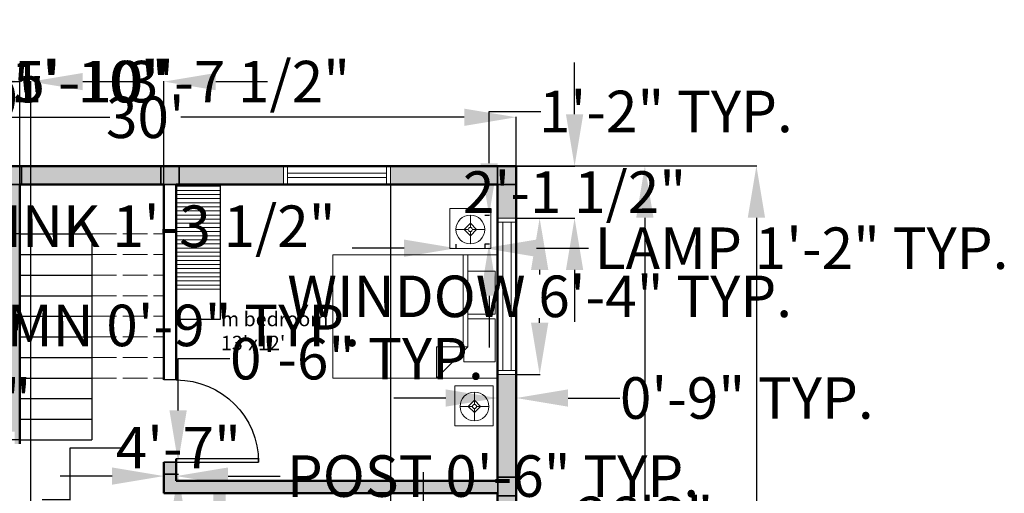
# Model space of a CAD drawing. Units: inches. Extents: x 25 to 82118, y 10 to 6494.
# Tile 8 of 9: x 40833 to 41311, y 3373 to 3603. Entities that reach past the tile are written whole.
import ezdxf

# ---------------------------------------------------------------- set-up
doc = ezdxf.new("R2010")
doc.units = ezdxf.units.IN
doc.header["$MEASUREMENT"] = 0
doc.linetypes.add('ACAD_ISO02W100', pattern=[15, 12, -3])
for name, color, linetype, lineweight in [('A-ANNO-DIMS', 2, 'Continuous', 18), ('A-AREA-IDEN', 7, 'Continuous', 25), ('A-DOOR', 3, 'Continuous', 25), ('A-FLOR-CASE', 8, 'Continuous', 25), ('A-FLOR-CASE-PATT', 9, 'Continuous', 13), ('A-FLOR-STRS', 7, 'Continuous', 25), ('A-FLOR-STRS-OVHD', 8, 'ACAD_ISO02W100', 18), ('A-FURN', 8, 'Continuous', 18), ('A-GLAZ', 4, 'Continuous', 18), ('A-WALL', 7, 'Continuous', 50)]:
    doc.layers.add(name, color=color, linetype=linetype, lineweight=lineweight)
doc.layers.add('A-COLS', color=30, linetype='Continuous', lineweight=35, true_color=0xf26722)
doc.layers.add('A-WALL-PATT', color=18, linetype='Continuous', lineweight=13, true_color=0x000000)
doc.styles.get("Standard").update_dxf_attribs({"font": 'arial.ttf'})
doc.dimstyles.get("Standard").update_dxf_attribs({"dimtxt": 20.18, "dimasz": 25.18, "dimexe": 0.18, "dimexo": 0.0625, "dimgap": 0.09, "dimtad": 0, "dimtih": 1, "dimtoh": 1, "dimdec": 0, "dimzin": 0, "dimdsep": 46, "dimlunit": 3, "dimtxsty": 'Standard', "dimcen": 0.09, "dimadec": 0, "dimazin": 0, "dimtfac": 1, "dimtdec": 0, "dimtofl": 0, "dimtmove": 0, "dimatfit": 3, "dimfxl": 1, "dimtolj": 1, "dimtzin": 0, "dimarcsym": 0})

# ---------------------------------------------------------------- blocks, each defined once
blk = doc.blocks.new('Bed - Queen')
for p, q in [((0, -80.00003), (0, 0)), ((0, 0), (59.99999, 0)), ((59.99999, 0), (59.99999, -80.00003)), ((7.99999, -1.2), (28.79998, -1.2)), ((7.99999, -14.4), (7.99999, -1.2)), ((28.79998, -1.2), (28.79998, -14.4)), ((31.19999, -1.2), (51.99999, -1.2)), ((31.19999, -14.4), (31.19999, -1.2)), ((51.99999, -1.2), (51.99999, -16.4)), ((0, -14.4), (44.8, -14.4)), ((44.8, -16.8), (0, -16.8)), ((59.99999, -29.6), (44.8, -14.4)), ((44.8, -14.4), (44.8, -29.6)), ((51.99999, -16.4), (46.79936, -16.4)), ((44.8, -29.6), (59.99999, -29.6)), ((59.99999, -80.00003), (0, -80.00003))]:
    blk.add_line(p, q)
blk = doc.blocks.new('Lamp - Table')
for p, q in [((0, 7), (0, 1)), ((-1, 0), (-7, 0)), ((0, 3), (-3, 0)), ((-3, 0), (0, -3)), ((3, 0), (0, 3)), ((0, -3), (3, 0)), ((1, 0), (7, 0)), ((0, -1), (0, -7))]:
    blk.add_line(p, q)
for radius in [7, 1]:
    blk.add_circle((0, 0), radius)
blk = doc.blocks.new('*U12')
for p, q in [((0, 0), (0, -6)), ((40, 0), (40, -6))]:
    blk.add_line(p, q)
blk.add_lwpolyline([(0, 0), (0, 40), (1.75, 40), (1.75, 0)], close=True)
blk.add_arc((0, 0), 40, 0, 90)
blk = doc.blocks.new('*D13')
at = {"layer": 'A-ANNO-DIMS', "color": 0, "lineweight": -2, "transparency": 16777216}
for p, q in [((40714.21, 3531.88), (40714.21, 3555.71)), ((40739.39, 3555.53), (40877, 3555.53)), ((41049.03, 3555.53), (40911.42, 3555.53)), ((41074.21, 3531.88), (41074.21, 3555.71))]:
    blk.add_line(p, q, dxfattribs=at)
at = {"layer": 'A-ANNO-DIMS', "color": 0, "transparency": 16777216}
for points in [[(40739.39, 3559.72), (40739.39, 3551.33), (40714.21, 3555.53)], [(41049.03, 3559.72), (41049.03, 3551.33), (41074.21, 3555.53)]]:
    blk.add_solid(points, dxfattribs=at)
at = {"layer": 'Defpoints', "color": 0, "transparency": 16777216}
for p in [(41074.21, 3555.53), (40714.21, 3531.82), (41074.21, 3531.82)]:
    blk.add_point(p, dxfattribs=at)
at = {"layer": 'A-ANNO-DIMS', "color": 0, "transparency": 16777216, "insert": (40894.21, 3555.53), "char_height": 20.18, "attachment_point": 5}
blk.add_mtext("\\A1;30'", dxfattribs=at)
blk = doc.blocks.new('*D15')
at = {"layer": 'A-ANNO-DIMS', "color": 0, "lineweight": -2, "transparency": 16777216}
for p, q in [((41074.27, 3531.88), (41136.86, 3531.88)), ((41136.68, 3506.7), (41136.68, 3371.51)), ((41136.68, 3215.52), (41136.68, 3350.71)), ((41074.27, 3190.34), (41136.86, 3190.34))]:
    blk.add_line(p, q, dxfattribs=at)
at = {"layer": 'A-ANNO-DIMS', "color": 0, "transparency": 16777216}
for points in [[(41132.48, 3506.7), (41140.87, 3506.7), (41136.68, 3531.88)], [(41132.48, 3215.52), (41140.87, 3215.52), (41136.68, 3190.34)]]:
    blk.add_solid(points, dxfattribs=at)
at = {"layer": 'Defpoints', "color": 0, "transparency": 16777216}
for p in [(41074.21, 3531.88), (41074.21, 3190.34), (41136.68, 3190.34)]:
    blk.add_point(p, dxfattribs=at)
at = {"layer": 'A-ANNO-DIMS', "color": 0, "transparency": 16777216, "insert": (41136.68, 3361.11), "char_height": 20.18, "attachment_point": 5}
blk.add_mtext('\\A1;26\'3"', dxfattribs=at)
blk = doc.blocks.new('*D16')
at = {"layer": 'A-ANNO-DIMS', "color": 0, "lineweight": -2, "transparency": 16777216}
for p, q in [((41074.33, 3531.88), (41191.01, 3531.88)), ((41190.83, 3506.7), (41190.83, 3350.25)), ((41190.83, 3173), (41190.83, 3329.45)), ((41074.33, 3147.82), (41191.01, 3147.82))]:
    blk.add_line(p, q, dxfattribs=at)
at = {"layer": 'A-ANNO-DIMS', "color": 0, "transparency": 16777216}
for points in [[(41186.63, 3506.7), (41195.02, 3506.7), (41190.83, 3531.88)], [(41186.63, 3173), (41195.02, 3173), (41190.83, 3147.82)]]:
    blk.add_solid(points, dxfattribs=at)
at = {"layer": 'Defpoints', "color": 0, "transparency": 16777216}
for p in [(41074.27, 3531.88), (41074.27, 3147.82), (41190.83, 3147.82)]:
    blk.add_point(p, dxfattribs=at)
at = {"layer": 'A-ANNO-DIMS', "color": 0, "transparency": 16777216, "insert": (41190.83, 3339.85), "char_height": 20.18, "attachment_point": 5}
blk.add_mtext("\\A1;32'", dxfattribs=at)
blk = doc.blocks.new('WIN-48IN-9W')
for p, q in [((0, 0), (0, 9)), ((2, 0), (2, 9)), ((2, 5.5), (50, 5.5)), ((50, 0), (50, 9)), ((52, 0), (52, 9)), ((2, 3.5), (50, 3.5))]:
    blk.add_line(p, q)
blk = doc.blocks.new('WIN-72IN-9W')
for p, q in [((9, 76), (0, 76)), ((9, 74), (0, 74)), ((2.5, 74), (2.5, 2)), ((6.5, 74), (6.5, 2)), ((9, 2), (0, 2)), ((9, 0), (0, 0))]:
    blk.add_line(p, q)
blk = doc.blocks.new('COL-9X9')
h = blk.add_hatch(color=256)
h.dxf.hatch_style = 1
h.paths.add_polyline_path([(9, 9), (0, 9), (0, 0), (9, 0)])
blk.add_lwpolyline([(0, 0), (9, 0), (9, 9), (0, 9)], close=True)
blk = doc.blocks.new('POST-INTERIOR-6IN')
h = blk.add_hatch(color=256)
h.dxf.hatch_style = 1
h.paths.add_polyline_path([(6, 5.8), (0, 5.8), (0, 0), (6, 0)])
blk.add_lwpolyline([(6, 5.8), (0, 5.8), (0, 0), (6, 0)], close=True)
blk = doc.blocks.new('*D25')
at = {"layer": 'A-ANNO-DIMS', "color": 0, "lineweight": -2, "transparency": 16777216}
for p, q in [((40724.56, 3429.21), (40724.56, 3454.39)), ((40724.56, 3454.39), (40749.74, 3454.39)), ((40723.27, 3404.03), (40724.74, 3404.03)), ((40723.27, 3395.03), (40724.74, 3395.03)), ((40724.56, 3369.85), (40724.56, 3344.67))]:
    blk.add_line(p, q, dxfattribs=at)
at = {"layer": 'A-ANNO-DIMS', "color": 0, "transparency": 16777216}
for points in [[(40720.36, 3429.21), (40728.76, 3429.21), (40724.56, 3404.03)], [(40720.36, 3369.85), (40728.76, 3369.85), (40724.56, 3395.03)]]:
    blk.add_solid(points, dxfattribs=at)
at = {"layer": 'Defpoints', "color": 0, "transparency": 16777216}
for p in [(40723.21, 3404.03), (40724.56, 3404.03), (40723.21, 3395.03)]:
    blk.add_point(p, dxfattribs=at)
at = {"layer": 'A-ANNO-DIMS', "color": 0, "transparency": 16777216, "insert": (40876.22, 3454.39), "char_height": 20.18, "attachment_point": 5}
blk.add_mtext('\\A1;COLUMN 0\'-9" TYP.', dxfattribs=at)
blk = doc.blocks.new('*D27')
at = {"layer": 'A-ANNO-DIMS', "color": 0, "lineweight": -2, "transparency": 16777216}
for p, q in [((40878.03, 3381.2), (40852.85, 3381.2)), ((40903.21, 3382.03), (40903.21, 3381.02)), ((40909.21, 3382.03), (40909.21, 3381.02)), ((40934.39, 3381.2), (40959.57, 3381.2))]:
    blk.add_line(p, q, dxfattribs=at)
at = {"layer": 'A-ANNO-DIMS', "color": 0, "transparency": 16777216}
for points in [[(40878.03, 3385.39), (40878.03, 3377), (40903.21, 3381.2)], [(40934.39, 3385.39), (40934.39, 3377), (40909.21, 3381.2)]]:
    blk.add_solid(points, dxfattribs=at)
at = {"layer": 'Defpoints', "color": 0, "transparency": 16777216}
for p in [(40903.21, 3382.1), (40909.21, 3382.1), (40909.21, 3381.2)]:
    blk.add_point(p, dxfattribs=at)
at = {"layer": 'A-ANNO-DIMS', "color": 0, "transparency": 16777216, "insert": (41062.95, 3381.2), "char_height": 20.18, "attachment_point": 5}
blk.add_mtext('\\A1;POST 0\'-6" TYP.', dxfattribs=at)
blk = doc.blocks.new('*D28')
at = {"layer": 'A-ANNO-DIMS', "color": 0, "lineweight": -2, "transparency": 16777216}
for p, q in [((40910.11, 3413.07), (40910.11, 3438.25)), ((40910.11, 3438.25), (40935.29, 3438.25)), ((40909.27, 3387.89), (40910.29, 3387.89)), ((40909.27, 3382.1), (40910.29, 3382.1)), ((40910.11, 3356.92), (40910.11, 3331.74))]:
    blk.add_line(p, q, dxfattribs=at)
at = {"layer": 'A-ANNO-DIMS', "color": 0, "transparency": 16777216}
for points in [[(40905.91, 3413.07), (40914.31, 3413.07), (40910.11, 3387.89)], [(40905.91, 3356.92), (40914.31, 3356.92), (40910.11, 3382.1)]]:
    blk.add_solid(points, dxfattribs=at)
at = {"layer": 'Defpoints', "color": 0, "transparency": 16777216}
for p in [(40909.21, 3387.89), (40910.11, 3387.89), (40909.21, 3382.1)]:
    blk.add_point(p, dxfattribs=at)
at = {"layer": 'A-ANNO-DIMS', "color": 0, "transparency": 16777216, "insert": (40996.88, 3438.25), "char_height": 20.18, "attachment_point": 5}
blk.add_mtext('\\A1;0\'-6" TYP.', dxfattribs=at)
blk = doc.blocks.new('*D29')
at = {"layer": 'A-ANNO-DIMS', "color": 0, "lineweight": -2, "transparency": 16777216}
for p, q in [((41074.27, 3506.52), (41085.79, 3506.52)), ((41085.61, 3481.34), (41085.61, 3479.06)), ((41085.61, 3455.7), (41085.61, 3457.99)), ((41074.27, 3430.52), (41085.79, 3430.52))]:
    blk.add_line(p, q, dxfattribs=at)
at = {"layer": 'A-ANNO-DIMS', "color": 0, "transparency": 16777216}
for points in [[(41081.41, 3481.34), (41089.81, 3481.34), (41085.61, 3506.52)], [(41081.41, 3455.7), (41089.81, 3455.7), (41085.61, 3430.52)]]:
    blk.add_solid(points, dxfattribs=at)
at = {"layer": 'Defpoints', "color": 0, "transparency": 16777216}
for p in [(41074.21, 3506.52), (41085.61, 3506.52), (41074.21, 3430.52)]:
    blk.add_point(p, dxfattribs=at)
at = {"layer": 'A-ANNO-DIMS', "color": 0, "transparency": 16777216, "insert": (41085.61, 3468.52), "char_height": 20.18, "attachment_point": 5}
blk.add_mtext('\\A1;WINDOW 6\'-4" TYP.', dxfattribs=at)
blk = doc.blocks.new('*D30')
at = {"layer": 'A-ANNO-DIMS', "color": 0, "lineweight": -2, "transparency": 16777216}
for p, q in [((41065.21, 3430.46), (41065.21, 3418.94)), ((41074.21, 3430.46), (41074.21, 3418.94)), ((41040.03, 3419.12), (41014.85, 3419.12)), ((41099.39, 3419.12), (41124.57, 3419.12))]:
    blk.add_line(p, q, dxfattribs=at)
at = {"layer": 'A-ANNO-DIMS', "color": 0, "transparency": 16777216}
for points in [[(41040.03, 3423.32), (41040.03, 3414.93), (41065.21, 3419.12)], [(41099.39, 3423.32), (41099.39, 3414.93), (41074.21, 3419.12)]]:
    blk.add_solid(points, dxfattribs=at)
at = {"layer": 'Defpoints', "color": 0, "transparency": 16777216}
for p in [(41065.21, 3430.52), (41074.21, 3430.52), (41074.21, 3419.12)]:
    blk.add_point(p, dxfattribs=at)
at = {"layer": 'A-ANNO-DIMS', "color": 0, "transparency": 16777216, "insert": (41186.16, 3419.12), "char_height": 20.18, "attachment_point": 5}
blk.add_mtext('\\A1;0\'-9" TYP.', dxfattribs=at)
blk = doc.blocks.new('*D33')
at = {"layer": 'A-ANNO-DIMS', "color": 0, "lineweight": -2, "transparency": 16777216}
for p, q in [((41044.96, 3493.94), (41044.96, 3491.72)), ((41058.96, 3493.94), (41058.96, 3491.72)), ((41019.78, 3491.9), (40994.6, 3491.9)), ((41084.14, 3491.9), (41109.32, 3491.9))]:
    blk.add_line(p, q, dxfattribs=at)
at = {"layer": 'A-ANNO-DIMS', "color": 0, "transparency": 16777216}
for points in [[(41019.78, 3496.1), (41019.78, 3487.71), (41044.96, 3491.9)], [(41084.14, 3496.1), (41084.14, 3487.71), (41058.96, 3491.9)]]:
    blk.add_solid(points, dxfattribs=at)
at = {"layer": 'Defpoints', "color": 0, "transparency": 16777216}
for p in [(41044.96, 3494), (41058.96, 3494), (41058.96, 3491.9)]:
    blk.add_point(p, dxfattribs=at)
at = {"layer": 'A-ANNO-DIMS', "color": 0, "transparency": 16777216, "insert": (41212.76, 3491.9), "char_height": 20.18, "attachment_point": 5}
blk.add_mtext('\\A1;LAMP 1\'-2" TYP.', dxfattribs=at)
blk = doc.blocks.new('*D34')
at = {"layer": 'A-ANNO-DIMS', "color": 0, "lineweight": -2, "transparency": 16777216}
for p, q in [((41061.06, 3533.18), (41061.06, 3558.36)), ((41061.06, 3558.36), (41086.24, 3558.36)), ((41059.02, 3508), (41061.24, 3508)), ((41059.02, 3494), (41061.24, 3494)), ((41061.06, 3468.82), (41061.06, 3443.64))]:
    blk.add_line(p, q, dxfattribs=at)
at = {"layer": 'A-ANNO-DIMS', "color": 0, "transparency": 16777216}
for points in [[(41056.86, 3533.18), (41065.25, 3533.18), (41061.06, 3508)], [(41056.86, 3468.82), (41065.25, 3468.82), (41061.06, 3494)]]:
    blk.add_solid(points, dxfattribs=at)
at = {"layer": 'Defpoints', "color": 0, "transparency": 16777216}
for p in [(41058.96, 3508), (41061.06, 3508), (41058.96, 3494)]:
    blk.add_point(p, dxfattribs=at)
at = {"layer": 'A-ANNO-DIMS', "color": 0, "transparency": 16777216, "insert": (41146.88, 3558.36), "char_height": 20.18, "attachment_point": 5}
blk.add_mtext('\\A1;1\'-2" TYP.', dxfattribs=at)
blk = doc.blocks.new('*D37')
at = {"layer": 'A-ANNO-DIMS', "color": 0, "lineweight": -2, "transparency": 16777216}
for p, q in [((40745.04, 3504.86), (40745.04, 3502.4)), ((40760.67, 3504.86), (40760.67, 3502.4)), ((40719.86, 3502.58), (40694.68, 3502.58)), ((40785.85, 3502.58), (40811.03, 3502.58))]:
    blk.add_line(p, q, dxfattribs=at)
at = {"layer": 'A-ANNO-DIMS', "color": 0, "transparency": 16777216}
for points in [[(40719.86, 3506.78), (40719.86, 3498.38), (40745.04, 3502.58)], [(40785.85, 3506.78), (40785.85, 3498.38), (40760.67, 3502.58)]]:
    blk.add_solid(points, dxfattribs=at)
at = {"layer": 'Defpoints', "color": 0, "transparency": 16777216}
for p in [(40745.04, 3504.92), (40760.67, 3504.92), (40760.67, 3502.58)]:
    blk.add_point(p, dxfattribs=at)
at = {"layer": 'A-ANNO-DIMS', "color": 0, "transparency": 16777216, "insert": (40898.22, 3502.58), "char_height": 20.18, "attachment_point": 5}
blk.add_mtext('\\A1;SINK 1\'-3 1/2"', dxfattribs=at)
blk = doc.blocks.new('*D38')
at = {"layer": 'A-ANNO-DIMS', "color": 0, "lineweight": -2, "transparency": 16777216}
for p, q in [((40763.01, 3539.22), (40763.01, 3564.4)), ((40763.01, 3564.4), (40788.19, 3564.4)), ((40760.73, 3514.04), (40763.19, 3514.04)), ((40760.73, 3504.92), (40763.19, 3504.92)), ((40763.01, 3479.74), (40763.01, 3454.56))]:
    blk.add_line(p, q, dxfattribs=at)
at = {"layer": 'A-ANNO-DIMS', "color": 0, "transparency": 16777216}
for points in [[(40758.81, 3539.22), (40767.21, 3539.22), (40763.01, 3514.04)], [(40758.81, 3479.74), (40767.21, 3479.74), (40763.01, 3504.92)]]:
    blk.add_solid(points, dxfattribs=at)
at = {"layer": 'Defpoints', "color": 0, "transparency": 16777216}
for p in [(40760.67, 3514.04), (40763.01, 3514.04), (40760.67, 3504.92)]:
    blk.add_point(p, dxfattribs=at)
at = {"layer": 'A-ANNO-DIMS', "color": 0, "transparency": 16777216, "insert": (40815.1, 3564.4), "char_height": 20.18, "attachment_point": 5}
blk.add_mtext('\\A1;0\'-9"', dxfattribs=at)
blk = doc.blocks.new('*D43')
at = {"layer": 'A-ANNO-DIMS', "color": 0, "lineweight": -2, "transparency": 16777216}
for p, q in [((41029.25, 3357.91), (41029.25, 3383.09)), ((41024.37, 3332.73), (41029.43, 3332.73)), ((41024.37, 3299.75), (41029.43, 3299.75)), ((41029.25, 3274.57), (41029.25, 3249.39))]:
    blk.add_line(p, q, dxfattribs=at)
at = {"layer": 'A-ANNO-DIMS', "color": 0, "transparency": 16777216}
for points in [[(41025.05, 3357.91), (41033.45, 3357.91), (41029.25, 3332.73)], [(41025.05, 3274.57), (41033.45, 3274.57), (41029.25, 3299.75)]]:
    blk.add_solid(points, dxfattribs=at)
at = {"layer": 'Defpoints', "color": 0, "transparency": 16777216}
for p in [(41024.3, 3332.73), (41029.25, 3332.73), (41024.3, 3299.75)]:
    blk.add_point(p, dxfattribs=at)
at = {"layer": 'A-ANNO-DIMS', "color": 0, "transparency": 16777216, "insert": (41029.25, 3316.24), "char_height": 20.18, "attachment_point": 5}
blk.add_mtext('\\A1;COFFEE TABLE 2\'-9"', dxfattribs=at)
blk = doc.blocks.new('*D48')
at = {"layer": 'A-ANNO-DIMS', "color": 0, "lineweight": -2, "transparency": 16777216}
for p, q in [((40857.74, 3369.8), (40857.74, 3394.98)), ((40857.74, 3394.98), (40882.92, 3394.98)), ((40844.15, 3369.8), (40857.92, 3369.8)), ((40857.74, 3339.98), (40857.74, 3344.62)), ((40844.15, 3314.8), (40857.92, 3314.8))]:
    blk.add_line(p, q, dxfattribs=at)
at = {"layer": 'A-ANNO-DIMS', "color": 0, "transparency": 16777216}
for points in [[(40853.54, 3344.62), (40861.93, 3344.62), (40857.74, 3369.8)], [(40853.54, 3339.98), (40861.93, 3339.98), (40857.74, 3314.8)]]:
    blk.add_solid(points, dxfattribs=at)
at = {"layer": 'Defpoints', "color": 0, "transparency": 16777216}
for p in [(40844.09, 3369.8), (40857.74, 3369.8), (40844.09, 3314.8)]:
    blk.add_point(p, dxfattribs=at)
at = {"layer": 'A-ANNO-DIMS', "color": 0, "transparency": 16777216, "insert": (40910.23, 3394.98), "char_height": 20.18, "attachment_point": 5}
blk.add_mtext('\\A1;4\'-7"', dxfattribs=at)
blk = doc.blocks.new('*D51')
at = {"layer": 'A-ANNO-DIMS', "color": 0, "lineweight": -2, "transparency": 16777216}
for p, q in [((40750.31, 3454.92), (40750.31, 3480.1)), ((40746.92, 3429.74), (40750.49, 3429.74)), ((40746.92, 3406.76), (40750.49, 3406.76)), ((40750.31, 3381.58), (40750.31, 3356.4))]:
    blk.add_line(p, q, dxfattribs=at)
at = {"layer": 'A-ANNO-DIMS', "color": 0, "transparency": 16777216}
for points in [[(40746.11, 3454.92), (40754.5, 3454.92), (40750.31, 3429.74)], [(40746.11, 3381.58), (40754.5, 3381.58), (40750.31, 3406.76)]]:
    blk.add_solid(points, dxfattribs=at)
at = {"layer": 'Defpoints', "color": 0, "transparency": 16777216}
for p in [(40746.86, 3429.74), (40750.31, 3429.74), (40746.86, 3406.76)]:
    blk.add_point(p, dxfattribs=at)
at = {"layer": 'A-ANNO-DIMS', "color": 0, "transparency": 16777216, "insert": (40750.31, 3418.25), "char_height": 20.18, "attachment_point": 5}
blk.add_mtext('\\A1;FRIDGE 1\'-11"', dxfattribs=at)
blk = doc.blocks.new('*D53')
at = {"layer": 'A-ANNO-DIMS', "color": 0, "lineweight": -2, "transparency": 16777216}
for p, q in [((40808.03, 3572.85), (40782.85, 3572.85)), ((40833.21, 3498.88), (40833.21, 3573.03)), ((40903.21, 3498.88), (40903.21, 3573.03)), ((40928.39, 3572.85), (40953.57, 3572.85))]:
    blk.add_line(p, q, dxfattribs=at)
at = {"layer": 'A-ANNO-DIMS', "color": 0, "transparency": 16777216}
for points in [[(40808.03, 3577.05), (40808.03, 3568.66), (40833.21, 3572.85)], [(40928.39, 3577.05), (40928.39, 3568.66), (40903.21, 3572.85)]]:
    blk.add_solid(points, dxfattribs=at)
at = {"layer": 'Defpoints', "color": 0, "transparency": 16777216}
for p in [(40903.21, 3572.85), (40833.21, 3498.82), (40903.21, 3498.82)]:
    blk.add_point(p, dxfattribs=at)
at = {"layer": 'A-ANNO-DIMS', "color": 0, "transparency": 16777216, "insert": (40868.21, 3572.85), "char_height": 20.18, "attachment_point": 5}
blk.add_mtext('\\A1;5\'-10"', dxfattribs=at)
blk = doc.blocks.new('*D54')
at = {"layer": 'A-ANNO-DIMS', "color": 0, "lineweight": -2, "transparency": 16777216}
for p, q in [((40833.15, 3498.82), (40804.83, 3498.82)), ((40805.01, 3473.64), (40805.01, 3459.21)), ((40805.01, 3424), (40805.01, 3438.43)), ((40833.15, 3398.82), (40804.83, 3398.82))]:
    blk.add_line(p, q, dxfattribs=at)
at = {"layer": 'A-ANNO-DIMS', "color": 0, "transparency": 16777216}
for points in [[(40800.81, 3473.64), (40809.21, 3473.64), (40805.01, 3498.82)], [(40800.81, 3424), (40809.21, 3424), (40805.01, 3398.82)]]:
    blk.add_solid(points, dxfattribs=at)
at = {"layer": 'Defpoints', "color": 0, "transparency": 16777216}
for p in [(40805.01, 3498.82), (40833.21, 3498.82), (40833.21, 3398.82)]:
    blk.add_point(p, dxfattribs=at)
at = {"layer": 'A-ANNO-DIMS', "color": 0, "transparency": 16777216, "insert": (40805.01, 3448.82), "char_height": 20.18, "attachment_point": 5}
blk.add_mtext('\\A1;8\'-4"', dxfattribs=at)
blk = doc.blocks.new('*D56')
at = {"layer": 'A-ANNO-DIMS', "color": 0, "lineweight": -2, "transparency": 16777216}
for p, q in [((40778.43, 3531.76), (40778.43, 3119.41)), ((40818.43, 3531.76), (40818.43, 3119.41)), ((40753.25, 3119.59), (40728.07, 3119.59)), ((40843.61, 3119.59), (40868.79, 3119.59))]:
    blk.add_line(p, q, dxfattribs=at)
at = {"layer": 'A-ANNO-DIMS', "color": 0, "transparency": 16777216}
for points in [[(40753.25, 3123.78), (40753.25, 3115.39), (40778.43, 3119.59)], [(40843.61, 3123.78), (40843.61, 3115.39), (40818.43, 3119.59)]]:
    blk.add_solid(points, dxfattribs=at)
at = {"layer": 'Defpoints', "color": 0, "transparency": 16777216}
for p in [(40778.43, 3531.82), (40818.43, 3531.82), (40818.43, 3119.59)]:
    blk.add_point(p, dxfattribs=at)
at = {"layer": 'A-ANNO-DIMS', "color": 0, "transparency": 16777216, "insert": (40895.69, 3119.59), "char_height": 20.18, "attachment_point": 5}
blk.add_mtext('\\A1;3\'-4"', dxfattribs=at)
blk = doc.blocks.new('*D58')
at = {"layer": 'A-ANNO-DIMS', "color": 0, "lineweight": -2, "transparency": 16777216}
for p, q in [((40735.53, 3572.85), (40710.35, 3572.85)), ((40760.71, 3246.88), (40760.71, 3573.03)), ((40782.73, 3246.88), (40782.73, 3573.03)), ((40807.91, 3572.85), (40833.09, 3572.85))]:
    blk.add_line(p, q, dxfattribs=at)
at = {"layer": 'A-ANNO-DIMS', "color": 0, "transparency": 16777216}
for points in [[(40735.53, 3577.05), (40735.53, 3568.66), (40760.71, 3572.85)], [(40807.91, 3577.05), (40807.91, 3568.66), (40782.73, 3572.85)]]:
    blk.add_solid(points, dxfattribs=at)
at = {"layer": 'Defpoints', "color": 0, "transparency": 16777216}
for p in [(40782.73, 3572.85), (40760.71, 3246.82), (40782.73, 3246.82)]:
    blk.add_point(p, dxfattribs=at)
at = {"layer": 'A-ANNO-DIMS', "color": 0, "transparency": 16777216, "insert": (40866.89, 3572.85), "char_height": 20.18, "attachment_point": 5}
blk.add_mtext('\\A1;1\'-10"', dxfattribs=at)
blk = doc.blocks.new('*D64')
at = {"layer": 'A-ANNO-DIMS', "color": 0, "lineweight": -2, "transparency": 16777216}
for p, q in [((41102.56, 3557), (41102.56, 3582.18)), ((41074.27, 3531.82), (41102.74, 3531.82)), ((41074.27, 3506.52), (41102.74, 3506.52)), ((41102.56, 3481.34), (41102.56, 3456.16))]:
    blk.add_line(p, q, dxfattribs=at)
at = {"layer": 'A-ANNO-DIMS', "color": 0, "transparency": 16777216}
for points in [[(41098.36, 3557), (41106.76, 3557), (41102.56, 3531.82)], [(41098.36, 3481.34), (41106.76, 3481.34), (41102.56, 3506.52)]]:
    blk.add_solid(points, dxfattribs=at)
at = {"layer": 'Defpoints', "color": 0, "transparency": 16777216}
for p in [(41074.21, 3531.82), (41102.56, 3531.82), (41074.21, 3506.52)]:
    blk.add_point(p, dxfattribs=at)
at = {"layer": 'A-ANNO-DIMS', "color": 0, "transparency": 16777216, "insert": (41102.56, 3519.17), "char_height": 20.18, "attachment_point": 5}
blk.add_mtext('\\A1;2\'-1 1/2"', dxfattribs=at)
blk = doc.blocks.new('*D66')
at = {"layer": 'A-ANNO-DIMS', "color": 0, "lineweight": -2, "transparency": 16777216}
for p, q in [((41013.21, 3522.76), (41013.21, 3119.41)), ((41065.21, 3522.76), (41065.21, 3119.41)), ((41038.39, 3119.59), (41040.03, 3119.59)), ((41065.21, 3119.59), (41090.39, 3119.59))]:
    blk.add_line(p, q, dxfattribs=at)
at = {"layer": 'A-ANNO-DIMS', "color": 0, "transparency": 16777216}
for points in [[(41038.39, 3123.78), (41038.39, 3115.39), (41013.21, 3119.59)], [(41040.03, 3123.78), (41040.03, 3115.39), (41065.21, 3119.59)]]:
    blk.add_solid(points, dxfattribs=at)
at = {"layer": 'Defpoints', "color": 0, "transparency": 16777216}
for p in [(41013.21, 3522.82), (41065.21, 3522.82), (41065.21, 3119.59)]:
    blk.add_point(p, dxfattribs=at)
at = {"layer": 'A-ANNO-DIMS', "color": 0, "transparency": 16777216, "insert": (41117.71, 3119.59), "char_height": 20.18, "attachment_point": 5}
blk.add_mtext('\\A1;4\'-4"', dxfattribs=at)
blk = doc.blocks.new('*D67')
at = {"layer": 'A-ANNO-DIMS', "color": 0, "lineweight": -2, "transparency": 16777216}
for p, q in [((40770.03, 3572.85), (40744.85, 3572.85)), ((40795.21, 3156.88), (40795.21, 3573.03)), ((40838.63, 3156.88), (40838.63, 3573.03)), ((40863.81, 3572.85), (40888.99, 3572.85))]:
    blk.add_line(p, q, dxfattribs=at)
at = {"layer": 'A-ANNO-DIMS', "color": 0, "transparency": 16777216}
for points in [[(40770.03, 3577.05), (40770.03, 3568.66), (40795.21, 3572.85)], [(40863.81, 3577.05), (40863.81, 3568.66), (40838.63, 3572.85)]]:
    blk.add_solid(points, dxfattribs=at)
at = {"layer": 'Defpoints', "color": 0, "transparency": 16777216}
for p in [(40838.63, 3572.85), (40795.21, 3156.82), (40838.63, 3156.82)]:
    blk.add_point(p, dxfattribs=at)
at = {"layer": 'A-ANNO-DIMS', "color": 0, "transparency": 16777216, "insert": (40939.41, 3572.85), "char_height": 20.18, "attachment_point": 5}
blk.add_mtext('\\A1;3\'-7 1/2"', dxfattribs=at)

msp = doc.modelspace()

# ---------------------------------------------------------------- hatches: boundary and pattern name
at = {"layer": 'A-FLOR-CASE-PATT'}
h = msp.add_hatch(dxfattribs=at)
h.set_pattern_fill('ANSI31', color=256, scale=16, angle=-45, style=0)
h.paths.add_polyline_path([(40909.5, 3470.2), (40930.51, 3470.2), (40930.51, 3522.2), (40909.5, 3522.2)])
at = {"layer": 'A-WALL-PATT'}
h = msp.add_hatch(color=256, dxfattribs=at)
h.dxf.hatch_style = 1
h.paths.add_polyline_path([(40778.43, 3531.82), (40723.21, 3531.82), (40723.21, 3522.82), (40778.54, 3522.82, -0.01877), (40778.43, 3525.82)])
h.paths.add_polyline_path([(40723.21, 3522.82), (40714.21, 3522.82), (40714.21, 3500.82), (40723.21, 3500.82)])
h.paths.add_polyline_path([(40723.21, 3424.82), (40714.21, 3424.82), (40714.21, 3404.03), (40723.21, 3404.03)])
h.paths.add_polyline_path([(40723.21, 3395.03), (40714.21, 3395.03), (40714.21, 3386.82), (40723.21, 3386.82)])
h.paths.add_polyline_path([(40901.65, 3531.82), (40834.16, 3531.82), (40834.16, 3522.82), (40901.65, 3522.82)])
h.paths.add_polyline_path([(40825.16, 3531.82), (40818.43, 3531.82), (40818.43, 3525.82), (40818.43, 3522.82), (40825.16, 3522.82)])
h.paths.add_polyline_path([(40961.21, 3531.82), (40910.65, 3531.82), (40910.65, 3522.82), (40961.21, 3522.82)])
h.paths.add_polyline_path([(41065.21, 3531.82), (41013.21, 3531.82), (41013.21, 3522.82), (41065.21, 3522.82)])
h.paths.add_polyline_path([(41074.21, 3522.82), (41065.21, 3522.82), (41065.21, 3506.52), (41074.21, 3506.52)])
h.paths.add_polyline_path([(41074.21, 3430.52), (41065.21, 3430.52), (41065.21, 3428.74), (41065.21, 3380.62), (41074.21, 3380.62)])
h.paths.add_polyline_path([(41074.21, 3371.62), (41065.21, 3371.62), (41065.21, 3355.41), (41074.21, 3355.41)])
h.paths.add_polyline_path([(41065.36, 3378.82), (40909.21, 3378.82), (40909.21, 3382.1), (40903.21, 3382.1), (40903.21, 3372.82), (41065.36, 3372.82)])
h.paths.add_polyline_path([(40933.21, 3372.82), (40927.21, 3372.82), (40927.21, 3282.62), (40933.21, 3282.62)])
h.paths.add_polyline_path([(41074.21, 3279.41), (41065.21, 3279.41), (41065.21, 3240.82), (41074.21, 3240.82)])
h.paths.add_polyline_path([(41065.21, 3246.82), (41052.05, 3246.82), (41052.05, 3240.82), (41065.21, 3240.82)])
h.paths.add_polyline_path([(40985.75, 3202.89), (41023.1, 3202.89), (41023.1, 3229.01), (40985.75, 3229.01)], flags=9)
h.paths.add_polyline_path([(40960.75, 3302.54), (40998.1, 3302.54), (40998.1, 3328.66), (40960.75, 3328.66)], flags=9)
h = msp.add_hatch(color=256, dxfattribs=at)
h.dxf.hatch_style = 1
h.paths.add_polyline_path([(40784.59, 3402.82), (40723.21, 3402.82), (40723.21, 3396.82), (40784.59, 3396.82)])
h.paths.add_polyline_path([(40833.21, 3522.82), (40827.21, 3522.82), (40827.21, 3402.75), (40830.71, 3402.75), (40830.71, 3396.82), (40833.21, 3396.82)])
h.paths.add_polyline_path([(40767.21, 3280.82), (40723.21, 3280.82), (40723.21, 3274.82), (40767.21, 3274.82)])
h.paths.add_polyline_path([(40723.21, 3288.82), (40714.21, 3288.82), (40714.21, 3283), (40723.21, 3283)])

# ---------------------------------------------------------------- linework, layer by layer
at = {"layer": 'A-FLOR-CASE'}
for p, q in [((40930.51, 3522.82), (40930.51, 3457.2)), ((40930.51, 3457.2), (40909.5, 3457.2))]:
    msp.add_line(p, q, dxfattribs=at)
at = {"layer": 'A-FLOR-STRS'}
for p, q in [((40833.21, 3498.82), (40868.21, 3498.82)), ((40868.21, 3498.82), (40868.21, 3398.82)), ((40833.21, 3488.82), (40868.21, 3488.82)), ((40833.21, 3478.82), (40868.21, 3478.82)), ((40833.21, 3468.82), (40868.21, 3468.82)), ((40833.21, 3458.82), (40868.21, 3458.82)), ((40833.21, 3448.82), (40868.21, 3448.82)), ((40833.21, 3438.82), (40868.21, 3438.82)), ((40833.21, 3438.82), (40868.21, 3438.82)), ((40833.21, 3428.82), (40868.21, 3428.82)), ((40833.21, 3418.82), (40868.21, 3418.82)), ((40833.21, 3408.82), (40868.21, 3408.82)), ((40833.21, 3398.82), (40868.21, 3398.82))]:
    msp.add_line(p, q, dxfattribs=at)
at = {"layer": 'A-FLOR-STRS-OVHD'}
for p, q in [((40868.21, 3498.82), (40903.21, 3498.82)), ((40868.21, 3488.82), (40903.21, 3488.82)), ((40868.21, 3478.82), (40903.21, 3478.82)), ((40868.21, 3468.82), (40903.21, 3468.82)), ((40868.21, 3458.82), (40903.21, 3458.82)), ((40868.21, 3448.82), (40903.21, 3448.82)), ((40868.21, 3438.82), (40903.21, 3438.82)), ((40868.21, 3428.82), (40903.21, 3428.82))]:
    msp.add_line(p, q, dxfattribs=at)
at = {"layer": 'A-FURN'}
for points in [[(41042, 3511.17), (41061.98, 3511.17), (41061.98, 3491.69), (41042, 3491.69)], [(41044.41, 3424.97), (41063.02, 3424.97), (41063.02, 3405.6), (41044.41, 3405.6)]]:
    msp.add_lwpolyline(points, close=True, dxfattribs=at)
at = {"layer": 'A-WALL'}
for p, q in [((40818.43, 3531.82), (41074.21, 3531.82)), ((41074.21, 3531.82), (41074.21, 3147.82)), ((40833.21, 3396.82), (40833.21, 3522.82)), ((40833.21, 3522.82), (40903.21, 3522.82)), ((40903.21, 3522.82), (40903.21, 3427.89)), ((40909.21, 3522.82), (40909.21, 3427.89)), ((40909.21, 3522.82), (41065.21, 3522.82)), ((41065.21, 3522.82), (41065.21, 3378.82)), ((40909.21, 3389.64), (40909.21, 3378.82)), ((40903.21, 3387.89), (40903.21, 3372.82)), ((40909.21, 3378.82), (41065.21, 3378.82)), ((40903.21, 3372.82), (41065.21, 3372.82)), ((41065.21, 3372.82), (41065.21, 3240.82))]:
    msp.add_line(p, q, dxfattribs=at)

# ---------------------------------------------------------------- block references
at = {"layer": 'A-COLS'}
for p, rotation in [((40834.16, 3522.82), 89.99999999996236), ((40910.65, 3522.82), 89.99999999996236), ((41074.21, 3522.82), 89.99999999991604), ((41074.36, 3371.62), 89.99999999995948)]:
    msp.add_blockref('COL-9X9', p, dxfattribs=dict(at, rotation=rotation))
msp.add_blockref('POST-INTERIOR-6IN', (40903.21, 3382.1), dxfattribs=at)
at = {"layer": 'A-DOOR', "xscale": -1, "rotation": 270}
msp.add_blockref('*U12', (40909.21, 3387.89), dxfattribs=at)
at = {"layer": 'A-FURN'}
for p in [(41051.96, 3501), (41053.97, 3415.02)]:
    msp.add_blockref('Lamp - Table', p, dxfattribs=at)
at = {"layer": 'A-FURN', "rotation": 270}
msp.add_blockref('Bed - Queen', (41065.21, 3488.74), dxfattribs=at)
at = {"layer": 'A-GLAZ'}
for name, p in [('WIN-48IN-9W', (40961.21, 3522.82)), ('WIN-72IN-9W', (41065.21, 3430.52))]:
    msp.add_blockref(name, p, dxfattribs=at)

# ---------------------------------------------------------------- texts
at = {"layer": 'A-AREA-IDEN', "insert": (40930.89, 3461.02), "char_height": 7, "attachment_point": 1}
msp.add_mtext_dynamic_manual_height_columns("m bedroom\\P13'x12'", width=132.9687, gutter_width=1, heights=[0], dxfattribs=at)

# ---------------------------------------------------------------- dimensions: what is measured, and where the dimension line sits
at = {"layer": 'A-ANNO-DIMS'}
for base, p1, p2, override, picture, middle in [((40838.63, 3572.85), (40795.21, 3156.82), (40838.63, 3156.82), {"dimdec": 1, "dimlfac": 1, "dimrnd": 0, "dimzin": 1, "dimdsep": 46, "dimlunit": 4, "dimfrac": 2}, '*D67', (40939.41, 3572.85)), ((40782.73, 3572.85), (40760.71, 3246.82), (40782.73, 3246.82), {"dimdec": 1, "dimlfac": 1, "dimrnd": 0, "dimzin": 1, "dimdsep": 46, "dimlunit": 4, "dimfrac": 2}, '*D58', (40866.89, 3572.85)), ((40903.21, 3572.85), (40833.21, 3498.82), (40903.21, 3498.82), {"dimdec": 1, "dimlfac": 1, "dimrnd": 0, "dimzin": 1, "dimdsep": 46, "dimlunit": 4, "dimfrac": 2}, '*D53', (40868.21, 3572.85)), ((41074.21, 3555.53), (40714.21, 3531.82), (41074.21, 3531.82), {"dimclrd": 0, "dimclre": 0, "dimclrt": 0}, '*D13', (40894.21, 3555.53)), ((40818.43, 3119.59), (40778.43, 3531.82), (40818.43, 3531.82), {"dimdec": 1, "dimlfac": 1, "dimrnd": 0, "dimzin": 1, "dimdsep": 46, "dimlunit": 4, "dimfrac": 2}, '*D56', (40895.69, 3119.59)), ((41065.21, 3119.59), (41013.21, 3522.82), (41065.21, 3522.82), {"dimdec": 1, "dimlfac": 1, "dimrnd": 0, "dimzin": 1, "dimdsep": 46, "dimlunit": 4, "dimfrac": 2}, '*D66', (41117.71, 3119.59))]:
    dim = msp.add_linear_dim(base=base, p1=p1, p2=p2, dimstyle='Standard', override=override, dxfattribs=at)
    dim.commit()
    dim.dimension.update_dxf_attribs({"geometry": picture, "text_midpoint": middle})
for base, p1, p2, text, override, picture, middle in [((41061.06, 3508), (41058.96, 3494), (41058.96, 3508), '<> TYP.', {"dimdec": 1, "dimlfac": 1, "dimrnd": 0, "dimzin": 1, "dimdsep": 46, "dimlunit": 4, "dimfrac": 2}, '*D34', (41146.88, 3558.36)), ((41136.68, 3190.34), (41074.21, 3531.88), (41074.21, 3190.34), '26\'3"', {"dimclrd": 0, "dimclre": 0, "dimclrt": 0}, '*D15', (41136.68, 3361.11)), ((41085.61, 3506.52), (41074.21, 3430.52), (41074.21, 3506.52), 'WINDOW <> TYP.', {"dimdec": 1, "dimlfac": 1, "dimrnd": 0, "dimzin": 1, "dimdsep": 46, "dimlunit": 4, "dimfrac": 2}, '*D29', (41085.61, 3468.52)), ((40724.56, 3404.03), (40723.21, 3395.03), (40723.21, 3404.03), 'COLUMN <> TYP.', {"dimdec": 1, "dimlfac": 1, "dimrnd": 0, "dimzin": 1, "dimdsep": 46, "dimlunit": 4, "dimfrac": 2}, '*D25', (40876.22, 3454.39)), ((40750.31, 3429.74), (40746.86, 3406.76), (40746.86, 3429.74), 'FRIDGE <>', {"dimdec": 1, "dimlfac": 1, "dimrnd": 0, "dimzin": 1, "dimdsep": 46, "dimlunit": 4, "dimfrac": 2}, '*D51', (40750.31, 3418.25)), ((40910.11, 3387.89), (40909.21, 3382.1), (40909.21, 3387.89), '<> TYP.', {"dimdec": 1, "dimlfac": 1, "dimrnd": 0, "dimzin": 1, "dimdsep": 46, "dimlunit": 4, "dimfrac": 2}, '*D28', (40996.88, 3438.25)), ((41029.25, 3332.73), (41024.3, 3299.75), (41024.3, 3332.73), 'COFFEE TABLE <>', {"dimdec": 1, "dimlfac": 1, "dimrnd": 0, "dimzin": 1, "dimdsep": 46, "dimlunit": 4, "dimfrac": 2}, '*D43', (41029.25, 3316.24))]:
    dim = msp.add_linear_dim(base=base, p1=p1, p2=p2, angle=90, text=text, dimstyle='Standard', override=override, dxfattribs=at)
    dim.commit()
    dim.dimension.update_dxf_attribs({"geometry": picture, "text_midpoint": middle})
for base, p1, p2, override, picture, middle in [((41102.56, 3531.82), (41074.21, 3506.52), (41074.21, 3531.82), {"dimdec": 1, "dimlfac": 1, "dimrnd": 0, "dimzin": 1, "dimdsep": 46, "dimlunit": 4, "dimfrac": 2}, '*D64', (41102.56, 3519.17)), ((40763.01, 3514.04), (40760.67, 3504.92), (40760.67, 3514.04), {"dimdec": 1, "dimlfac": 1, "dimrnd": 0, "dimzin": 1, "dimdsep": 46, "dimlunit": 4, "dimfrac": 2}, '*D38', (40815.1, 3564.4)), ((41190.83, 3147.82), (41074.27, 3531.88), (41074.27, 3147.82), {"dimclrd": 0, "dimclre": 0, "dimclrt": 0}, '*D16', (41190.83, 3339.85)), ((40805.01, 3498.82), (40833.21, 3398.82), (40833.21, 3498.82), {"dimdec": 1, "dimlfac": 1, "dimrnd": 0, "dimzin": 1, "dimdsep": 46, "dimlunit": 4, "dimfrac": 2}, '*D54', (40805.01, 3448.82)), ((40857.74, 3369.8), (40844.09, 3314.8), (40844.09, 3369.8), {"dimdec": 1, "dimlfac": 1, "dimrnd": 0, "dimzin": 1, "dimdsep": 46, "dimlunit": 4, "dimfrac": 2}, '*D48', (40910.23, 3394.98))]:
    dim = msp.add_linear_dim(base=base, p1=p1, p2=p2, angle=90, dimstyle='Standard', override=override, dxfattribs=at)
    dim.commit()
    dim.dimension.update_dxf_attribs({"geometry": picture, "text_midpoint": middle})
for base, p1, p2, text, picture, middle in [((40760.67, 3502.58), (40745.04, 3504.92), (40760.67, 3504.92), 'SINK <>', '*D37', (40898.22, 3502.58)), ((41058.96, 3491.9), (41044.96, 3494), (41058.96, 3494), 'LAMP <> TYP.', '*D33', (41212.76, 3491.9)), ((41074.21, 3419.12), (41065.21, 3430.52), (41074.21, 3430.52), '<> TYP.', '*D30', (41186.16, 3419.12)), ((40909.21, 3381.2), (40903.21, 3382.1), (40909.21, 3382.1), 'POST <> TYP.', '*D27', (41062.95, 3381.2))]:
    dim = msp.add_linear_dim(base=base, p1=p1, p2=p2, text=text, dimstyle='Standard', override={"dimdec": 1, "dimlfac": 1, "dimrnd": 0, "dimzin": 1, "dimdsep": 46, "dimlunit": 4, "dimfrac": 2}, dxfattribs=at)
    dim.commit()
    dim.dimension.update_dxf_attribs({"geometry": picture, "text_midpoint": middle})

doc.saveas('drawing.dxf')
